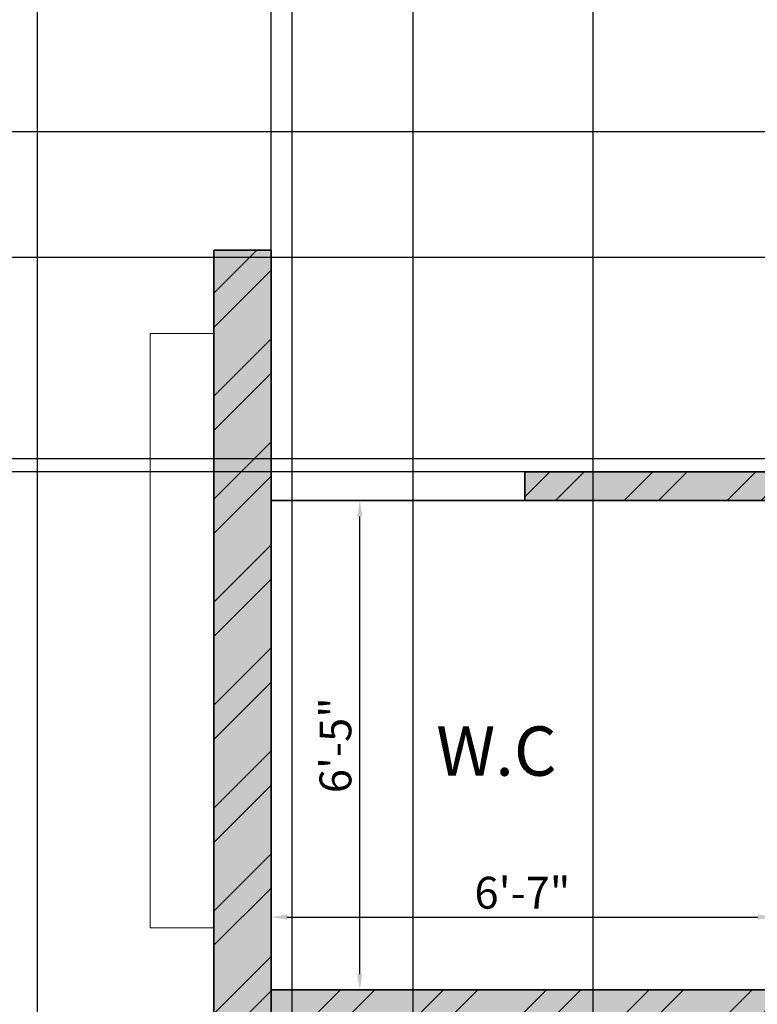
# Model space of a CAD drawing. Units: inches. Extents: x 1804 to 3296, y 909 to 2477.
# Tile 13 of 31: x 2119 to 2235, y 1329 to 1484. Entities that reach past the tile are written whole.
import ezdxf

# ---------------------------------------------------------------- set-up
doc = ezdxf.new("R2010")
doc.units = ezdxf.units.IN
for name, color, linetype, lineweight in [('A-ANNO-DIMS', 2, 'Continuous', 18), ('A-ANNO-TTLB', 156, 'Continuous', 35), ('A-AREA-IDEN', 190, 'Continuous', 18), ('A-WALL-PATT', 10, 'Continuous', 13), ('FUR', 100, 'Continuous', 18), ('WALL', 10, 'Continuous', 35)]:
    doc.layers.add(name, color=color, linetype=linetype, lineweight=lineweight)
doc.styles.get("Standard").update_dxf_attribs({"font": 'arial.ttf'})
doc.dimstyles.new('ISO-25', dxfattribs={"dimtxt": 5, "dimasz": 2.5, "dimexe": 1.25, "dimexo": 0.625, "dimtad": 1, "dimdec": 0, "dimlunit": 4, "dimtxsty": 'Standard', "dimcen": 2.5, "dimadec": 0, "dimazin": 0, "dimtfac": 1, "dimtdec": 0, "dimtmove": 0, "dimatfit": 3, "dimfxl": 1, "dimarcsym": 0})
pattern_1 = [(45, (0, 196.207), (-8.08223, 8.08223), []), (45, (5.388, 196.207), (-8.08223, 8.08223), [])]

# ---------------------------------------------------------------- blocks, each defined once
blk = doc.blocks.new('*D16')
at = {"layer": 'A-ANNO-DIMS', "color": 0, "lineweight": -2, "transparency": 16777216}
for p, q in [((2158.58, 1331.82), (2158.58, 1343.89)), ((2237.56, 1331.82), (2237.56, 1343.89)), ((2161.08, 1342.64), (2235.06, 1342.64))]:
    blk.add_line(p, q, dxfattribs=at)
at = {"layer": 'A-ANNO-DIMS', "color": 0, "lineweight": 100, "transparency": 16777216}
for points in [[(2161.08, 1343.05), (2161.08, 1342.22), (2158.58, 1342.64)], [(2235.06, 1343.05), (2235.06, 1342.22), (2237.56, 1342.64)]]:
    blk.add_solid(points, dxfattribs=at)
at = {"layer": 'Defpoints', "color": 0, "lineweight": 100, "transparency": 16777216}
for p in [(2237.56, 1342.64), (2158.58, 1331.19), (2237.56, 1331.19)]:
    blk.add_point(p, dxfattribs=at)
at = {"layer": 'A-ANNO-DIMS', "color": 0, "transparency": 16777216, "insert": (2198.07, 1345.81), "char_height": 5, "attachment_point": 5}
blk.add_mtext('6\'-7"', dxfattribs=at)
blk = doc.blocks.new('*D17')
at = {"layer": 'A-ANNO-DIMS', "color": 0, "lineweight": -2, "transparency": 16777216}
for p, q in [((2159.2, 1408.06), (2173.77, 1408.06)), ((2172.52, 1333.69), (2172.52, 1405.56)), ((2159.2, 1331.19), (2173.77, 1331.19))]:
    blk.add_line(p, q, dxfattribs=at)
at = {"layer": 'A-ANNO-DIMS', "color": 0, "lineweight": 100, "transparency": 16777216}
for points in [[(2172.1, 1405.56), (2172.93, 1405.56), (2172.52, 1408.06)], [(2172.1, 1333.69), (2172.93, 1333.69), (2172.52, 1331.19)]]:
    blk.add_solid(points, dxfattribs=at)
at = {"layer": 'Defpoints', "color": 0, "lineweight": 100, "transparency": 16777216}
for p in [(2158.58, 1408.06), (2172.52, 1408.06), (2158.58, 1331.19)]:
    blk.add_point(p, dxfattribs=at)
at = {"layer": 'A-ANNO-DIMS', "color": 0, "transparency": 16777216, "insert": (2169.34, 1369.63), "char_height": 5, "attachment_point": 5, "rotation": 90}
blk.add_mtext('6\'-5"', dxfattribs=at)
blk = doc.blocks.new('*D56')
at = {"layer": 'A-ANNO-DIMS', "color": 0, "lineweight": -2, "transparency": 16777216}
for p, q in [((2180.87, 1680.42), (2180.87, 975.89)), ((2268, 1680.42), (2268, 975.89)), ((2183.37, 977.14), (2265.5, 977.14))]:
    blk.add_line(p, q, dxfattribs=at)
at = {"layer": 'A-ANNO-DIMS', "color": 0, "lineweight": 100, "transparency": 16777216}
for points in [[(2183.37, 977.56), (2183.37, 976.72), (2180.87, 977.14)], [(2265.5, 977.56), (2265.5, 976.72), (2268, 977.14)]]:
    blk.add_solid(points, dxfattribs=at)
at = {"layer": 'Defpoints', "color": 0, "lineweight": 100, "transparency": 16777216}
for p in [(2180.87, 1681.04), (2268, 1681.04), (2268, 977.14)]:
    blk.add_point(p, dxfattribs=at)
at = {"layer": 'A-ANNO-DIMS', "color": 0, "transparency": 16777216, "insert": (2224.44, 980.32), "char_height": 5, "attachment_point": 5}
blk.add_mtext('7\'-3"', dxfattribs=at)
blk = doc.blocks.new('*D59')
at = {"layer": 'A-ANNO-DIMS', "color": 0, "lineweight": -2, "transparency": 16777216}
for p, q in [((2121.83, 1590.3), (2121.83, 975.89)), ((2161.83, 1590.3), (2161.83, 975.89)), ((2124.33, 977.14), (2159.33, 977.14))]:
    blk.add_line(p, q, dxfattribs=at)
at = {"layer": 'A-ANNO-DIMS', "color": 0, "lineweight": 100, "transparency": 16777216}
for points in [[(2124.33, 977.56), (2124.33, 976.72), (2121.83, 977.14)], [(2159.33, 977.56), (2159.33, 976.72), (2161.83, 977.14)]]:
    blk.add_solid(points, dxfattribs=at)
at = {"layer": 'Defpoints', "color": 0, "lineweight": 100, "transparency": 16777216}
for p in [(2121.83, 1590.92), (2161.83, 1590.92), (2161.83, 977.14)]:
    blk.add_point(p, dxfattribs=at)
at = {"layer": 'A-ANNO-DIMS', "color": 0, "transparency": 16777216, "insert": (2141.83, 980.32), "char_height": 5, "attachment_point": 5}
blk.add_mtext('3\'-4"', dxfattribs=at)
blk = doc.blocks.new('*D64')
at = {"layer": 'A-ANNO-DIMS', "color": 0, "lineweight": -2, "transparency": 16777216}
for p, q in [((2241.43, 1446.21), (1880.63, 1446.21)), ((1881.88, 1417.08), (1881.88, 1443.71)), ((2241.43, 1414.58), (1880.63, 1414.58))]:
    blk.add_line(p, q, dxfattribs=at)
at = {"layer": 'A-ANNO-DIMS', "color": 0, "lineweight": 100, "transparency": 16777216}
for points in [[(1881.47, 1443.71), (1882.3, 1443.71), (1881.88, 1446.21)], [(1881.47, 1417.08), (1882.3, 1417.08), (1881.88, 1414.58)]]:
    blk.add_solid(points, dxfattribs=at)
at = {"layer": 'Defpoints', "color": 0, "lineweight": 100, "transparency": 16777216}
for p in [(1881.88, 1446.21), (2242.06, 1446.21), (2242.06, 1414.58)]:
    blk.add_point(p, dxfattribs=at)
at = {"layer": 'A-ANNO-DIMS', "color": 0, "transparency": 16777216, "insert": (1878.67, 1430.39), "char_height": 5, "attachment_point": 5, "rotation": 90}
blk.add_mtext('2\'-7 1/2"', dxfattribs=at)
blk = doc.blocks.new('*D66')
at = {"layer": 'A-ANNO-DIMS', "color": 0, "lineweight": -2, "transparency": 16777216}
for p, q in [((2282.03, 1465.94), (1880.63, 1465.94)), ((1881.88, 1415.06), (1881.88, 1463.44)), ((2282.03, 1412.56), (1880.63, 1412.56))]:
    blk.add_line(p, q, dxfattribs=at)
at = {"layer": 'A-ANNO-DIMS', "color": 0, "lineweight": 100, "transparency": 16777216}
for points in [[(1881.47, 1463.44), (1882.3, 1463.44), (1881.88, 1465.94)], [(1881.47, 1415.06), (1882.3, 1415.06), (1881.88, 1412.56)]]:
    blk.add_solid(points, dxfattribs=at)
at = {"layer": 'Defpoints', "color": 0, "lineweight": 100, "transparency": 16777216}
for p in [(1881.88, 1465.94), (2282.65, 1465.94), (2282.65, 1412.56)]:
    blk.add_point(p, dxfattribs=at)
at = {"layer": 'A-ANNO-DIMS', "color": 0, "transparency": 16777216, "insert": (1878.67, 1439.25), "char_height": 5, "attachment_point": 5, "rotation": 90}
blk.add_mtext('4\'-5 1/2"', dxfattribs=at)
blk = doc.blocks.new('*D71')
at = {"layer": 'A-ANNO-DIMS', "color": 0, "lineweight": -2, "transparency": 16777216}
for p, q in [((2158.58, 1272.26), (2158.58, 1874.99)), ((2161.08, 1873.74), (2206.69, 1873.74)), ((2209.19, 1272.26), (2209.19, 1874.99))]:
    blk.add_line(p, q, dxfattribs=at)
at = {"layer": 'A-ANNO-DIMS', "color": 0, "lineweight": 100, "transparency": 16777216}
for points in [[(2161.08, 1874.15), (2161.08, 1873.32), (2158.58, 1873.74)], [(2206.69, 1874.15), (2206.69, 1873.32), (2209.19, 1873.74)]]:
    blk.add_solid(points, dxfattribs=at)
at = {"layer": 'Defpoints', "color": 0, "lineweight": 100, "transparency": 16777216}
for p in [(2209.19, 1873.74), (2158.58, 1271.63), (2209.19, 1271.63)]:
    blk.add_point(p, dxfattribs=at)
at = {"layer": 'A-ANNO-DIMS', "color": 0, "transparency": 16777216, "insert": (2183.88, 1876.95), "char_height": 5, "attachment_point": 5}
blk.add_mtext('4\'-2 1/2"', dxfattribs=at)

msp = doc.modelspace()

# ---------------------------------------------------------------- hatches: boundary and pattern name
at = {"layer": 'A-ANNO-TTLB'}
h = msp.add_hatch(color=256, dxfattribs=at)
h.dxf.hatch_style = 1
h.paths.add_polyline_path([(3294.53, 2476.54), (1803.79, 2476.54), (1805.43, 909.47), (3296.17, 909.47)])
h.paths.add_polyline_path([(1811, 914.33), (1812.79, 2467.54), (3285.53, 2467.54), (3283.74, 914.33)], flags=16)
h.paths.add_polyline_path([(1925.58, 1062.77), (1925.58, 1138.07), (1925.58, 1539.88), (1925.58, 1793.38), (1925.58, 1830.04), (2325.54, 1830.04), (2325.54, 1793.38), (2325.54, 1586.42), (2325.54, 1138.07), (2325.54, 1062.77)], flags=0)
h.paths.add_polyline_path([(1997.22, 1029.4), (2008.85, 1037.96), (2008.85, 1020.84)], flags=0)
h.paths.add_polyline_path([(1934.58, 1138.07), (1934.58, 1147.07), (2078.77, 1147.07), (2078.77, 1138.07), (2060.94, 1138.07)], flags=0)
h.paths.add_polyline_path([(1944.35, 1138.07), (1944.35, 1147.07), (2056.05, 1147.07), (2056.05, 1138.07)], flags=0)
h.paths.add_polyline_path([(2222.24, 1037.96), (2233.87, 1029.4), (2222.24, 1020.84)], flags=0)
h.paths.add_polyline_path([(2061.94, 1139.07), (2061.94, 1146.07), (2077.77, 1146.07), (2077.77, 1139.07)], flags=0)
h.paths.add_polyline_path([(2149.58, 1138.07), (2149.58, 1269.44), (2158.58, 1269.44), (2158.58, 1326.69), (2149.58, 1326.69), (2149.58, 1340.94), (2139.6, 1340.94), (2139.6, 1434.25), (2149.58, 1434.25), (2149.58, 1447.36), (2158.58, 1447.36), (2158.58, 1423.87), (2158.58, 1408.06), (2198.46, 1408.06), (2198.46, 1412.56), (2282.65, 1412.56), (2282.65, 1465.94), (2316.54, 1465.94), (2316.54, 1590.92), (2192.86, 1590.92), (2192.86, 1595.3), (2291.17, 1595.3), (2291.17, 1590.92), (2316.54, 1590.92), (2316.54, 1784.38), (2300.24, 1784.38), (2300.24, 1757.47), (2268, 1757.47), (2268, 1681.04), (2180.87, 1681.04), (2180.87, 1757.47), (2148.63, 1757.47), (2148.63, 1784.38), (2119.08, 1784.38), (2119.08, 1585.58), (2114.58, 1585.58), (2114.58, 1784.38), (2064.11, 1784.38), (2046.28, 1784.38), (2046.28, 1760.38), (1958.58, 1760.38), (1958.58, 1664.38), (1934.58, 1664.38), (1934.58, 1784.38), (1934.58, 1793.38), (2046.28, 1793.38), (2064.11, 1793.38), (2119.08, 1793.38), (2230.78, 1793.38), (2230.78, 1784.38), (2268, 1784.38), (2300.24, 1784.38), (2316.54, 1784.38), (2316.54, 1590.92), (2316.54, 1373.73), (2316.54, 1138.07)], flags=0)
h.paths.add_polyline_path([(2209.19, 1166.63), (2209.19, 1175.63), (2158.58, 1175.63), (2209.19, 1223.63), (2209.19, 1231.63), (2183.88, 1231.63), (2183.88, 1301.66), (2242.59, 1301.66), (2242.59, 1326.69), (2316.54, 1326.69), (2272.59, 1271.63), (2272.59, 1223.63), (2316.54, 1175.63), (2272.59, 1175.63), (2272.59, 1166.63)], flags=0)
h.paths.add_polyline_path([(1947.77, 1345.22), (1947.77, 1457.48), (1991.2, 1457.48), (1991.2, 1451.7), (1991.2, 1352.18), (1991.2, 1345.22)], flags=0)
h.paths.add_polyline_path([(2209.19, 1271.63), (2262.59, 1271.63), (2262.59, 1311.85), (2272.59, 1301.66), (2272.59, 1271.63), (2269.92, 1269.63), (2270.59, 1269.63), (2270.59, 1225.63), (2211.19, 1225.63), (2211.19, 1269.63), (2211.86, 1269.63)], flags=0)
h.paths.add_polyline_path([(2000.34, 1378.21), (2000.34, 1429.71), (2025.22, 1429.71), (2025.22, 1378.21)], flags=0)
h.paths.add_polyline_path([(2001.34, 1379.21), (2001.34, 1428.71), (2024.22, 1428.71), (2024.22, 1379.21)], flags=0)
h.paths.add_polyline_path([(2012.34, 1390.21), (2012.34, 1417.71), (2013.22, 1417.71), (2013.22, 1390.21)], flags=0)
h.paths.add_polyline_path([(2237.56, 1331.19), (2237.56, 1340.18), (2238.62, 1340.18), (2238.62, 1386.84), (2241.04, 1386.84), (2242.06, 1386.84), (2242.06, 1408.06), (2316.54, 1331.19)], flags=0)
h.paths.add_polyline_path([(1953.73, 1464.35), (1953.73, 1498.59), (1981.74, 1498.59), (1981.74, 1464.35)], flags=0)
h.paths.add_polyline_path([(1987.63, 1462.08), (1987.63, 1500.95), (2104.07, 1500.95), (2104.07, 1462.08), (2099.27, 1462.08), (1993.6, 1462.08)], flags=0)
h.paths.add_polyline_path([(1956.06, 1481.47, -1), (1979.41, 1481.47, -1)], flags=0)
edge = h.paths.add_edge_path(flags=0)
edge.add_ellipse((2299.53, 1438.37), major_axis=(0.31, 21.36), ratio=0.670333, start_angle=0, end_angle=360)
h.paths.add_polyline_path([(2297.39, 1438.37, -1), (2301.67, 1438.37, -1)], flags=0)
h.paths.add_polyline_path([(2591.54, 1163.23), (2591.54, 1179.38), (2591.54, 1379.68), (2591.54, 1395.84), (2734.5, 1395.84), (2734.5, 1379.68), (2734.5, 1179.38), (2734.5, 1163.23)], flags=0)
h.paths.add_polyline_path([(2592.54, 1164.23), (2592.54, 1166.23), (2733.5, 1166.23), (2733.5, 1164.23)], flags=0)
h.paths.add_polyline_path([(2592.54, 1180.38), (2592.54, 1378.68), (2733.5, 1378.68), (2733.5, 1180.38)], flags=0)
h.paths.add_polyline_path([(2593.54, 1181.38), (2593.54, 1377.68), (2732.5, 1377.68), (2732.5, 1181.38)], flags=0)
h.paths.add_polyline_path([(2594.54, 1182.38), (2594.54, 1376.68), (2731.5, 1376.68), (2731.5, 1182.38)], flags=0)
h.paths.add_polyline_path([(1936.95, 1697.46), (1936.95, 1736.46), (1955.41, 1736.46), (1955.41, 1697.46)], flags=0)
h.paths.add_polyline_path([(1938.48, 1718.36), (1938.48, 1734.92), (1953.65, 1734.92), (1953.65, 1718.36)], flags=0)
h.paths.add_polyline_path([(1944.75, 1726.64, -1), (1947.37, 1726.64, -1)], flags=0)
h.paths.add_polyline_path([(2592.54, 1394.84), (2733.5, 1394.84), (2733.5, 1392.84), (2592.54, 1392.84)], flags=0)
h.paths.add_polyline_path([(1976.61, 1762.5), (1976.61, 1781.44), (2012.79, 1781.44), (2012.79, 1762.5)], flags=0)
h.paths.add_polyline_path([(1979.57, 1771.97, -1), (1991.39, 1771.97, -1)], flags=0)
h.paths.add_polyline_path([(1995.36, 1771.97, -1), (2007.18, 1771.97, -1)], flags=0)
h.paths.add_polyline_path([(2251.51, 1744.53), (2268, 1730.05), (2251.51, 1730.05)], flags=0)
h.paths.add_polyline_path([(2047.28, 1785.38), (2047.28, 1792.38), (2063.11, 1792.38), (2063.11, 1785.38)], flags=0)
h.paths.add_polyline_path([(2155.08, 1770.92, -1), (2174.42, 1770.92, -1)], flags=0)
h.paths.add_polyline_path([(2188.59, 1758.27), (2188.59, 1772.81), (2222.3, 1772.81), (2222.3, 1758.27)], flags=0)
h.paths.add_polyline_path([(2223.97, 1758.27), (2223.97, 1772.81), (2257.68, 1772.81), (2257.68, 1758.27)], flags=0)
h.paths.add_polyline_path([(2274.45, 1770.92, -1), (2293.8, 1770.92, -1)], flags=0)
h.paths.add_polyline_path([(2591.54, 1582.09), (2591.54, 1782.39), (2734.5, 1782.39), (2734.5, 1582.09)], flags=0)
h.paths.add_polyline_path([(2592.54, 1583.09), (2592.54, 1781.39), (2733.5, 1781.39), (2733.5, 1583.09)], flags=0)
h.paths.add_polyline_path([(2593.54, 1584.09), (2593.54, 1780.39), (2732.5, 1780.39), (2732.5, 1584.09)], flags=0)
h.paths.add_polyline_path([(2594.54, 1585.09), (2594.54, 1779.39), (2731.5, 1779.39), (2731.5, 1585.09)], flags=0)
h.paths.add_polyline_path([(1922.17, 1978.79), (1922.17, 2295.08), (1922.17, 2296.08), (2115.67, 2296.08), (2115.67, 2384.31), (2115.67, 2385.31), (2322.12, 2385.31), (2323.12, 2385.31), (2323.12, 1979.79), (2323.12, 1978.79), (1923.17, 1978.79)], flags=0)
h.paths.add_polyline_path([(1922.17, 1978.79), (1922.17, 2051.31), (1922.17, 2214.86), (1922.17, 2296.08), (2115.67, 2296.08), (2115.67, 2385.31), (2323.12, 2385.31), (2323.12, 2280.42), (2323.12, 1978.79), (2115.67, 1978.79)], flags=0)
h.paths.add_polyline_path([(1923.17, 1979.79), (1923.17, 2050.31), (2115.67, 2050.31), (2115.67, 2051.31), (1923.17, 2051.31), (1923.17, 2213.86), (1923.17, 2214.86), (1923.17, 2295.08), (1990.02, 2295.08), (1990.02, 2214.86), (1991.02, 2214.86), (1991.02, 2295.08), (2115.67, 2295.08), (2115.67, 1979.79), (2116.67, 1979.79), (2116.67, 2304.18), (2116.67, 2384.31), (2322.12, 2384.31), (2322.12, 2280.42), (2322.12, 1979.79), (2115.67, 1979.79)], flags=0)
h.paths.add_polyline_path([(2972.46, 1192.5), (2972.46, 1196.92), (2995.47, 1196.92), (2995.47, 1255.47), (2995.09, 1255.47), (2987.42, 1249.39), (2980.08, 1255.47), (2978.05, 1255.47), (2978.05, 1257.24), (2995.47, 1257.24), (2995.47, 1261.58), (3015.37, 1261.58), (3015.37, 1333.28), (3015.37, 1414.4), (3032.82, 1414.4), (3032.82, 1333.28), (3032.82, 1261.58), (3052.66, 1261.58), (3052.66, 1255.47), (3079.86, 1255.47), (3078.72, 1254.57), (3081.47, 1252.29), (3078.56, 1249.99), (3075.81, 1252.26), (3072.57, 1249.69), (3070.36, 1251.52), (3067.67, 1249.39), (3060.34, 1255.47), (3052.66, 1255.47), (3052.66, 1196.92), (3054.58, 1196.92), (3074, 1196.92), (3074, 1192.5), (3052.66, 1192.5), (2995.47, 1192.5)], flags=0)
h.paths.add_polyline_path([(2490.75, 1979.27), (2490.75, 1980.27), (2596.87, 1980.27), (2596.87, 2051.8), (2596.87, 2052.8), (2596.87, 2216.35), (2596.87, 2297.57), (2717.32, 2297.57), (2710.57, 2305.62), (2724.07, 2305.62), (2717.32, 2297.57), (2782.37, 2297.57), (2782.37, 2395.8), (3006.82, 2395.8), (3006.82, 1981.27), (3093.73, 1981.27), (3093.73, 1980.27), (3047.51, 1980.27), (3046.37, 1979.37), (3049.11, 1977.1), (3046.2, 1974.79), (3043.46, 1977.07), (3040.21, 1974.49), (3038, 1976.32), (3035.32, 1974.2), (3027.98, 1980.27), (2871.83, 1980.27), (2871.83, 1981.27), (2791.37, 1981.27), (2791.37, 2050.8), (2597.87, 2050.8), (2597.87, 1980.27), (2597.87, 1979.27), (2546.27, 1979.27), (2545.12, 1978.37), (2547.87, 1976.1), (2544.96, 1973.79), (2542.22, 1976.07), (2538.97, 1973.49), (2536.76, 1975.32), (2534.07, 1973.2), (2526.74, 1979.27)], flags=0)
h.paths.add_polyline_path([(2597.87, 2051.8), (2606.87, 2051.8), (2606.87, 2258.39), (2597.87, 2258.39), (2597.87, 2296.57), (2606.87, 2296.57), (2606.87, 2262.39), (2782.37, 2262.39), (2782.37, 2296.57), (2790.37, 2296.57), (2790.37, 2262.39), (2791.37, 2262.39), (2791.37, 2305.67), (2791.37, 2385.8), (2996.82, 2385.8), (2996.82, 2339.85), (3006.82, 2339.85), (3006.82, 2250.12), (2997.82, 2250.12), (2997.82, 1981.27), (2996.82, 1981.27), (2872.83, 1981.27), (2872.83, 1991.8), (2871.83, 1991.8), (2871.83, 2050.8), (2790.37, 2050.8), (2597.87, 2050.8)], flags=0)
h.paths.add_polyline_path([(2179.93, 2153.92), (2179.93, 2353.97), (2259.98, 2353.97), (2259.98, 2153.92)], flags=0)
h.paths.add_polyline_path([(2180.93, 2154.92), (2180.93, 2352.97), (2258.98, 2352.97), (2258.98, 2154.92)], flags=0)
h.paths.add_polyline_path([(2960.87, 1608.49), (2960.87, 1753.62), (3070.9, 1753.62), (3070.9, 1608.49)], flags=0)
h.paths.add_polyline_path([(2961.87, 1609.49), (2961.87, 1752.62), (3069.9, 1752.62), (3069.9, 1609.49)], flags=0)
h.paths.add_polyline_path([(2962.87, 1610.49), (2962.87, 1751.62), (3068.9, 1751.62), (3068.9, 1610.49)], flags=0)
h.paths.add_polyline_path([(2963.87, 1611.49), (2963.87, 1750.62), (3067.9, 1750.62), (3067.9, 1611.49)], flags=0)
h.paths.add_polyline_path([(2782.37, 2051.8), (2782.37, 2216.32), (2791.37, 2216.32), (2791.37, 2051.8), (2872.83, 2051.8), (2872.83, 2068.56), (2884.67, 2068.56), (2884.67, 2085.33), (2896.51, 2085.33), (2896.51, 2102.09), (2908.36, 2102.09), (2908.36, 2118.85), (2920.2, 2118.85), (2920.2, 2135.62), (2932.05, 2135.62), (2932.05, 2145.3), (2925.08, 2145.3), (2925.08, 2203.2), (2996.82, 2203.2), (2996.82, 2145.3), (2953.82, 2145.3), (2872.83, 2051.8), (2790.37, 2051.8)], flags=0)
h.paths.add_polyline_path([(2717.32, 2238.65), (2710.57, 2246.7), (2724.07, 2246.7)], flags=0)
h.paths.add_polyline_path([(2003.09, 1122.79), (2017.16, 1122.79), (2017.16, 1138.74), (2003.09, 1138.74)], flags=8)
h.paths.add_polyline_path([(2174.76, 1792.72), (2188.83, 1792.72), (2188.83, 1808.66), (2174.76, 1808.66)], flags=8)
h.paths.add_polyline_path([(1987.95, 1792.51), (2002.02, 1792.51), (2002.02, 1808.45), (1987.95, 1808.45)], flags=8)
h.paths.add_polyline_path([(2148.79, 1289.26), (2160.46, 1289.26), (2160.46, 1305.2), (2148.79, 1305.2)], flags=8)
h.paths.add_polyline_path([(2115.36, 1133.57), (2127.04, 1133.57), (2127.04, 1149.51), (2115.36, 1149.51)], flags=8)
h.paths.add_polyline_path([(2237.58, 1421.48), (2249.25, 1421.48), (2249.25, 1437.43), (2237.58, 1437.43)], flags=8)
h.paths.add_polyline_path([(2134.99, 1584.32), (2146.66, 1584.32), (2146.66, 1600.26), (2134.99, 1600.26)], flags=8)
h.paths.add_polyline_path([(2101.95, 1557.31), (2113.62, 1557.31), (2113.62, 1573.25), (2101.95, 1573.25)], flags=8)
h.paths.add_polyline_path([(2937.85, 1156.77), (3120.41, 1156.77), (3120.41, 1185.72), (2937.85, 1185.72)], flags=8)
h.paths.add_polyline_path([(2980.71, 1786.71), (3050.06, 1786.71), (3050.06, 1802.66), (2980.71, 1802.66)], flags=8)
h.paths.add_polyline_path([(2869.28, 1661.96), (2938.62, 1661.96), (2938.62, 1690.8), (2869.28, 1690.8)], flags=8)
h.paths.add_polyline_path([(3092.27, 1674.86), (3161.62, 1674.86), (3161.62, 1690.8), (3092.27, 1690.8)], flags=8)
h.paths.add_polyline_path([(2980.71, 1674.86), (3050.06, 1674.86), (3050.06, 1690.8), (2980.71, 1690.8)], flags=8)
h.paths.add_polyline_path([(2649.07, 1678.23), (2674.53, 1678.23), (2674.53, 1714.76), (2649.07, 1714.76)], flags=8)
h.paths.add_polyline_path([(2530.84, 1981.63), (2549.13, 1981.63), (2549.13, 1997.57), (2530.84, 1997.57)], flags=8)
h.paths.add_polyline_path([(3031.29, 1981.77), (3049.58, 1981.77), (3049.58, 1997.71), (3031.29, 1997.71)], flags=8)
h.paths.add_polyline_path([(2715.38, 1911.9), (2851.54, 1911.9), (2851.54, 1940.85), (2715.38, 1940.85)], flags=8)
h.paths.add_polyline_path([(2015.23, 1927.36), (2205.42, 1927.36), (2205.42, 1956.3), (2015.23, 1956.3)], flags=8)
h.paths.add_polyline_path([(2671.84, 2057.84), (2702.75, 2057.84), (2702.75, 2073.79), (2671.84, 2073.79)], flags=8)
h.paths.add_polyline_path([(2678.5, 2316.52), (2765.26, 2316.52), (2765.26, 2332.46), (2678.5, 2332.46)], flags=8)
h.paths.add_polyline_path([(2678.48, 2271.96), (2736.41, 2271.96), (2736.41, 2287.9), (2678.48, 2287.9)], flags=8)
h.paths.add_polyline_path([(2019.2, 972.79), (2243.21, 972.79), (2243.21, 1001.74), (2019.2, 1001.74)], flags=8)
h.paths.add_polyline_path([(2097.06, 1021.56), (2132.16, 1021.56), (2132.16, 1037.51), (2097.06, 1037.51)], flags=8)
h.paths.add_polyline_path([(2182.47, 1360.48), (2207.35, 1360.48), (2207.35, 1376.42), (2182.47, 1376.42)], flags=8)
h.paths.add_polyline_path([(2261.12, 1361.77), (2295.01, 1361.77), (2295.01, 1377.71), (2261.12, 1377.71)], flags=8)
h.paths.add_polyline_path([(2245.75, 1511.51), (2278.44, 1511.51), (2278.44, 1527.46), (2245.75, 1527.46)], flags=8)
h.paths.add_polyline_path([(1991.16, 1296.29), (2060.51, 1296.29), (2060.51, 1312.23), (1991.16, 1312.23)], flags=8)
h.paths.add_polyline_path([(2187, 1651.35), (2246.71, 1651.35), (2246.71, 1667.29), (2187, 1667.29)], flags=8)
h.paths.add_polyline_path([(1976.49, 1684.81), (2068.63, 1684.81), (2068.63, 1700.76), (1976.49, 1700.76)], flags=8)
at = {"layer": 'A-WALL-PATT'}
h = msp.add_hatch(color=256, dxfattribs=at)
h.dxf.hatch_style = 1
h.paths.add_polyline_path([(2119.08, 1544.38), (1925.58, 1544.38), (1925.58, 1539.88), (2119.08, 1539.88)])
h.paths.add_polyline_path([(2119.08, 1545.58), (2114.58, 1545.58), (2114.58, 1544.38), (2119.08, 1544.38)])
h.paths.add_polyline_path([(1965.87, 1658.79), (1965.87, 1679.09), (1955.57, 1679.09), (1955.57, 1658.79)], flags=9)
h.paths.add_polyline_path([(2293.18, 1677.29), (2293.18, 1697.58), (2282.88, 1697.58), (2282.88, 1677.29)], flags=9)
h.paths.add_polyline_path([(2271.13, 1545.23), (2287.53, 1545.23), (2287.53, 1555.53), (2271.13, 1555.53)], flags=9)
h.paths.add_polyline_path([(2303.26, 1488.52), (2303.26, 1508.82), (2292.95, 1508.82), (2292.95, 1488.52)], flags=9)
h.paths.add_polyline_path([(2271.13, 1393.15), (2287.53, 1393.15), (2287.53, 1403.45), (2271.13, 1403.45)], flags=9)
h.paths.add_polyline_path([(2306.48, 1361.45), (2306.48, 1377.86), (2296.18, 1377.86), (2296.18, 1361.45)], flags=9)
h.paths.add_polyline_path([(2174.54, 1361.45), (2174.54, 1377.86), (2164.23, 1377.86), (2164.23, 1361.45)], flags=9)
h.paths.add_polyline_path([(1968.21, 1333.34), (1968.21, 1353.64), (1957.91, 1353.64), (1957.91, 1333.34)], flags=9)
h.paths.add_polyline_path([(2003.09, 1122.79), (2017.16, 1122.79), (2017.16, 1138.74), (2003.09, 1138.74)], flags=9)
h.paths.add_polyline_path([(2174.76, 1792.72), (2188.83, 1792.72), (2188.83, 1808.66), (2174.76, 1808.66)], flags=9)
h.paths.add_polyline_path([(1987.95, 1792.51), (2002.02, 1792.51), (2002.02, 1808.45), (1987.95, 1808.45)], flags=9)
h.paths.add_polyline_path([(2148.79, 1289.26), (2160.46, 1289.26), (2160.46, 1305.2), (2148.79, 1305.2)], flags=9)
h.paths.add_polyline_path([(2115.36, 1133.57), (2127.04, 1133.57), (2127.04, 1149.51), (2115.36, 1149.51)], flags=9)
h.paths.add_polyline_path([(2237.58, 1421.48), (2249.25, 1421.48), (2249.25, 1437.43), (2237.58, 1437.43)], flags=9)
h.paths.add_polyline_path([(2134.99, 1584.32), (2146.66, 1584.32), (2146.66, 1600.26), (2134.99, 1600.26)], flags=9)
h.paths.add_polyline_path([(2101.95, 1557.31), (2113.62, 1557.31), (2113.62, 1573.25), (2101.95, 1573.25)], flags=9)
h.paths.add_polyline_path([(2937.85, 1156.77), (3120.41, 1156.77), (3120.41, 1185.72), (2937.85, 1185.72)], flags=9)
h.paths.add_polyline_path([(2980.71, 1786.71), (3050.06, 1786.71), (3050.06, 1802.66), (2980.71, 1802.66)], flags=9)
h.paths.add_polyline_path([(2869.28, 1661.96), (2938.62, 1661.96), (2938.62, 1690.8), (2869.28, 1690.8)], flags=9)
h.paths.add_polyline_path([(3092.27, 1674.86), (3161.62, 1674.86), (3161.62, 1690.8), (3092.27, 1690.8)], flags=9)
h.paths.add_polyline_path([(2980.71, 1674.86), (3050.06, 1674.86), (3050.06, 1690.8), (2980.71, 1690.8)], flags=9)
h.paths.add_polyline_path([(2649.07, 1678.23), (2674.53, 1678.23), (2674.53, 1714.76), (2649.07, 1714.76)], flags=9)
h.paths.add_polyline_path([(2530.84, 1981.63), (2549.13, 1981.63), (2549.13, 1997.57), (2530.84, 1997.57)], flags=9)
h.paths.add_polyline_path([(3031.29, 1981.77), (3049.58, 1981.77), (3049.58, 1997.71), (3031.29, 1997.71)], flags=9)
h.paths.add_polyline_path([(2715.38, 1911.9), (2851.54, 1911.9), (2851.54, 1940.85), (2715.38, 1940.85)], flags=9)
h.paths.add_polyline_path([(2015.23, 1927.36), (2205.42, 1927.36), (2205.42, 1956.3), (2015.23, 1956.3)], flags=9)
h.paths.add_polyline_path([(2671.84, 2057.84), (2702.75, 2057.84), (2702.75, 2073.79), (2671.84, 2073.79)], flags=9)
h.paths.add_polyline_path([(2678.5, 2316.52), (2765.26, 2316.52), (2765.26, 2332.46), (2678.5, 2332.46)], flags=9)
h.paths.add_polyline_path([(2678.48, 2271.96), (2736.41, 2271.96), (2736.41, 2287.9), (2678.48, 2287.9)], flags=9)
h.paths.add_polyline_path([(2019.2, 972.79), (2243.21, 972.79), (2243.21, 1001.74), (2019.2, 1001.74)], flags=9)
h.paths.add_polyline_path([(2097.06, 1021.56), (2132.16, 1021.56), (2132.16, 1037.51), (2097.06, 1037.51)], flags=9)
h.paths.add_polyline_path([(2182.47, 1360.48), (2207.35, 1360.48), (2207.35, 1376.42), (2182.47, 1376.42)], flags=9)
h.paths.add_polyline_path([(2261.12, 1361.77), (2295.01, 1361.77), (2295.01, 1377.71), (2261.12, 1377.71)], flags=9)
h.paths.add_polyline_path([(2245.75, 1511.51), (2278.44, 1511.51), (2278.44, 1527.46), (2245.75, 1527.46)], flags=9)
h.paths.add_polyline_path([(1991.16, 1296.29), (2060.51, 1296.29), (2060.51, 1312.23), (1991.16, 1312.23)], flags=9)
h.paths.add_polyline_path([(2187, 1651.35), (2246.71, 1651.35), (2246.71, 1667.29), (2187, 1667.29)], flags=9)
h.paths.add_polyline_path([(1976.49, 1684.81), (2068.63, 1684.81), (2068.63, 1700.76), (1976.49, 1700.76)], flags=9)
h = msp.add_hatch(color=256, dxfattribs=at)
h.dxf.hatch_style = 1
h.paths.add_polyline_path([(2149.58, 1147.07), (2141.21, 1147.07), (2141.21, 1144.07), (2141.21, 1138.07), (2149.58, 1138.07)])
h.paths.add_polyline_path([(2101.21, 1144.07, -0.01877), (2101.32, 1147.07), (2078.77, 1147.07), (2078.77, 1138.07), (2101.21, 1138.07)])
h.paths.add_polyline_path([(2060.94, 1147.07), (2056.05, 1147.07), (2056.05, 1138.07), (2060.94, 1138.07)])
h.paths.add_polyline_path([(1944.35, 1147.07), (1934.58, 1147.07), (1934.58, 1138.07), (1944.35, 1138.07)])
h.paths.add_polyline_path([(2158.58, 1269.44), (2149.58, 1269.44), (2149.58, 1138.07), (2158.58, 1138.07)])
h.paths.add_polyline_path([(2003.09, 1122.79), (2017.16, 1122.79), (2017.16, 1138.74), (2003.09, 1138.74)], flags=9)
h.paths.add_polyline_path([(2174.76, 1792.72), (2188.83, 1792.72), (2188.83, 1808.66), (2174.76, 1808.66)], flags=9)
h.paths.add_polyline_path([(1987.95, 1792.51), (2002.02, 1792.51), (2002.02, 1808.45), (1987.95, 1808.45)], flags=9)
h.paths.add_polyline_path([(2148.79, 1289.26), (2160.46, 1289.26), (2160.46, 1305.2), (2148.79, 1305.2)], flags=9)
h.paths.add_polyline_path([(2115.36, 1133.57), (2127.04, 1133.57), (2127.04, 1149.51), (2115.36, 1149.51)], flags=9)
h.paths.add_polyline_path([(2237.58, 1421.48), (2249.25, 1421.48), (2249.25, 1437.43), (2237.58, 1437.43)], flags=9)
h.paths.add_polyline_path([(2134.99, 1584.32), (2146.66, 1584.32), (2146.66, 1600.26), (2134.99, 1600.26)], flags=9)
h.paths.add_polyline_path([(2101.95, 1557.31), (2113.62, 1557.31), (2113.62, 1573.25), (2101.95, 1573.25)], flags=9)
h.paths.add_polyline_path([(2937.85, 1156.77), (3120.41, 1156.77), (3120.41, 1185.72), (2937.85, 1185.72)], flags=9)
h.paths.add_polyline_path([(2980.71, 1786.71), (3050.06, 1786.71), (3050.06, 1802.66), (2980.71, 1802.66)], flags=9)
h.paths.add_polyline_path([(2869.28, 1661.96), (2938.62, 1661.96), (2938.62, 1690.8), (2869.28, 1690.8)], flags=9)
h.paths.add_polyline_path([(3092.27, 1674.86), (3161.62, 1674.86), (3161.62, 1690.8), (3092.27, 1690.8)], flags=9)
h.paths.add_polyline_path([(2980.71, 1674.86), (3050.06, 1674.86), (3050.06, 1690.8), (2980.71, 1690.8)], flags=9)
h.paths.add_polyline_path([(2649.07, 1678.23), (2674.53, 1678.23), (2674.53, 1714.76), (2649.07, 1714.76)], flags=9)
h.paths.add_polyline_path([(2530.84, 1981.63), (2549.13, 1981.63), (2549.13, 1997.57), (2530.84, 1997.57)], flags=9)
h.paths.add_polyline_path([(3031.29, 1981.77), (3049.58, 1981.77), (3049.58, 1997.71), (3031.29, 1997.71)], flags=9)
h.paths.add_polyline_path([(2715.38, 1911.9), (2851.54, 1911.9), (2851.54, 1940.85), (2715.38, 1940.85)], flags=9)
h.paths.add_polyline_path([(2015.23, 1927.36), (2205.42, 1927.36), (2205.42, 1956.3), (2015.23, 1956.3)], flags=9)
h.paths.add_polyline_path([(2671.84, 2057.84), (2702.75, 2057.84), (2702.75, 2073.79), (2671.84, 2073.79)], flags=9)
h.paths.add_polyline_path([(2678.5, 2316.52), (2765.26, 2316.52), (2765.26, 2332.46), (2678.5, 2332.46)], flags=9)
h.paths.add_polyline_path([(2678.48, 2271.96), (2736.41, 2271.96), (2736.41, 2287.9), (2678.48, 2287.9)], flags=9)
h.paths.add_polyline_path([(2019.2, 972.79), (2243.21, 972.79), (2243.21, 1001.74), (2019.2, 1001.74)], flags=9)
h.paths.add_polyline_path([(2097.06, 1021.56), (2132.16, 1021.56), (2132.16, 1037.51), (2097.06, 1037.51)], flags=9)
h.paths.add_polyline_path([(2182.47, 1360.48), (2207.35, 1360.48), (2207.35, 1376.42), (2182.47, 1376.42)], flags=9)
h.paths.add_polyline_path([(2261.12, 1361.77), (2295.01, 1361.77), (2295.01, 1377.71), (2261.12, 1377.71)], flags=9)
h.paths.add_polyline_path([(2245.75, 1511.51), (2278.44, 1511.51), (2278.44, 1527.46), (2245.75, 1527.46)], flags=9)
h.paths.add_polyline_path([(1991.16, 1296.29), (2060.51, 1296.29), (2060.51, 1312.23), (1991.16, 1312.23)], flags=9)
h.paths.add_polyline_path([(2187, 1651.35), (2246.71, 1651.35), (2246.71, 1667.29), (2187, 1667.29)], flags=9)
h.paths.add_polyline_path([(1976.49, 1684.81), (2068.63, 1684.81), (2068.63, 1700.76), (1976.49, 1700.76)], flags=9)
h = msp.add_hatch(color=256, dxfattribs=at)
h.dxf.hatch_style = 1
h.paths.add_polyline_path([(2158.58, 1275.49), (2155.29, 1275.49), (2149.58, 1275.49), (2149.58, 1269.44), (2158.58, 1269.44)])
h.paths.add_polyline_path([(2158.58, 1326.69), (2149.58, 1326.69), (2149.58, 1319.33), (2155.29, 1319.33), (2158.58, 1319.33)])
h.paths.add_polyline_path([(2158.58, 1402.2), (2158.58, 1423.87), (2158.58, 1447.36), (2149.58, 1447.36), (2149.58, 1423.87), (2149.58, 1340.94), (2149.58, 1326.69), (2158.58, 1326.69), (2158.58, 1354.23)])
h.paths.add_polyline_path([(1965.87, 1658.79), (1965.87, 1679.09), (1955.57, 1679.09), (1955.57, 1658.79)], flags=9)
h.paths.add_polyline_path([(2293.18, 1677.29), (2293.18, 1697.58), (2282.88, 1697.58), (2282.88, 1677.29)], flags=9)
h.paths.add_polyline_path([(2271.13, 1545.23), (2287.53, 1545.23), (2287.53, 1555.53), (2271.13, 1555.53)], flags=9)
h.paths.add_polyline_path([(2303.26, 1488.52), (2303.26, 1508.82), (2292.95, 1508.82), (2292.95, 1488.52)], flags=9)
h.paths.add_polyline_path([(2271.13, 1393.15), (2287.53, 1393.15), (2287.53, 1403.45), (2271.13, 1403.45)], flags=9)
h.paths.add_polyline_path([(2306.48, 1361.45), (2306.48, 1377.86), (2296.18, 1377.86), (2296.18, 1361.45)], flags=9)
h.paths.add_polyline_path([(2189.9, 1340.62), (2206.31, 1340.62), (2206.31, 1350.92), (2189.9, 1350.92)], flags=9)
h.paths.add_polyline_path([(2174.54, 1361.45), (2174.54, 1377.86), (2164.23, 1377.86), (2164.23, 1361.45)], flags=9)
h.paths.add_polyline_path([(2304.24, 1240.8), (2304.24, 1261.09), (2293.94, 1261.09), (2293.94, 1240.8)], flags=9)
h.paths.add_polyline_path([(2227.19, 1188.73), (2247.49, 1188.73), (2247.49, 1199.03), (2227.19, 1199.03)], flags=9)
h.paths.add_polyline_path([(2181.93, 1144.21), (2181.93, 1160.62), (2171.63, 1160.62), (2171.63, 1144.21)], flags=9)
h.paths.add_polyline_path([(1968.21, 1333.34), (1968.21, 1353.64), (1957.91, 1353.64), (1957.91, 1333.34)], flags=9)
h.paths.add_polyline_path([(2029.78, 1203.53), (2053.95, 1203.53), (2053.95, 1213.83), (2029.78, 1213.83)], flags=9)
h.paths.add_polyline_path([(2576.51, 1671.88), (2576.51, 1692.17), (2566.21, 1692.17), (2566.21, 1671.88)], flags=9)
h.paths.add_polyline_path([(2566.99, 1269.67), (2566.99, 1289.96), (2556.68, 1289.96), (2556.68, 1269.67)], flags=9)
h.paths.add_polyline_path([(2581.85, 1269.17), (2581.85, 1289.46), (2571.54, 1289.46), (2571.54, 1269.17)], flags=9)
h.paths.add_polyline_path([(2650.71, 1409.75), (2674.89, 1409.75), (2674.89, 1420.05), (2650.71, 1420.05)], flags=9)
h.paths.add_polyline_path([(2003.09, 1122.79), (2017.16, 1122.79), (2017.16, 1138.74), (2003.09, 1138.74)], flags=9)
h.paths.add_polyline_path([(2174.76, 1792.72), (2188.83, 1792.72), (2188.83, 1808.66), (2174.76, 1808.66)], flags=9)
h.paths.add_polyline_path([(1987.95, 1792.51), (2002.02, 1792.51), (2002.02, 1808.45), (1987.95, 1808.45)], flags=9)
h.paths.add_polyline_path([(2148.79, 1289.26), (2160.46, 1289.26), (2160.46, 1305.2), (2148.79, 1305.2)], flags=9)
h.paths.add_polyline_path([(2115.36, 1133.57), (2127.04, 1133.57), (2127.04, 1149.51), (2115.36, 1149.51)], flags=9)
h.paths.add_polyline_path([(2237.58, 1421.48), (2249.25, 1421.48), (2249.25, 1437.43), (2237.58, 1437.43)], flags=9)
h.paths.add_polyline_path([(2134.99, 1584.32), (2146.66, 1584.32), (2146.66, 1600.26), (2134.99, 1600.26)], flags=9)
h.paths.add_polyline_path([(2101.95, 1557.31), (2113.62, 1557.31), (2113.62, 1573.25), (2101.95, 1573.25)], flags=9)
h.paths.add_polyline_path([(2937.85, 1156.77), (3120.41, 1156.77), (3120.41, 1185.72), (2937.85, 1185.72)], flags=9)
h.paths.add_polyline_path([(2980.71, 1786.71), (3050.06, 1786.71), (3050.06, 1802.66), (2980.71, 1802.66)], flags=9)
h.paths.add_polyline_path([(2869.28, 1661.96), (2938.62, 1661.96), (2938.62, 1690.8), (2869.28, 1690.8)], flags=9)
h.paths.add_polyline_path([(3092.27, 1674.86), (3161.62, 1674.86), (3161.62, 1690.8), (3092.27, 1690.8)], flags=9)
h.paths.add_polyline_path([(2980.71, 1674.86), (3050.06, 1674.86), (3050.06, 1690.8), (2980.71, 1690.8)], flags=9)
h.paths.add_polyline_path([(2649.07, 1678.23), (2674.53, 1678.23), (2674.53, 1714.76), (2649.07, 1714.76)], flags=9)
h.paths.add_polyline_path([(2530.84, 1981.63), (2549.13, 1981.63), (2549.13, 1997.57), (2530.84, 1997.57)], flags=9)
h.paths.add_polyline_path([(3031.29, 1981.77), (3049.58, 1981.77), (3049.58, 1997.71), (3031.29, 1997.71)], flags=9)
h.paths.add_polyline_path([(2715.38, 1911.9), (2851.54, 1911.9), (2851.54, 1940.85), (2715.38, 1940.85)], flags=9)
h.paths.add_polyline_path([(2015.23, 1927.36), (2205.42, 1927.36), (2205.42, 1956.3), (2015.23, 1956.3)], flags=9)
h.paths.add_polyline_path([(2671.84, 2057.84), (2702.75, 2057.84), (2702.75, 2073.79), (2671.84, 2073.79)], flags=9)
h.paths.add_polyline_path([(2678.5, 2316.52), (2765.26, 2316.52), (2765.26, 2332.46), (2678.5, 2332.46)], flags=9)
h.paths.add_polyline_path([(2678.48, 2271.96), (2736.41, 2271.96), (2736.41, 2287.9), (2678.48, 2287.9)], flags=9)
h.paths.add_polyline_path([(2019.2, 972.79), (2243.21, 972.79), (2243.21, 1001.74), (2019.2, 1001.74)], flags=9)
h.paths.add_polyline_path([(2097.06, 1021.56), (2132.16, 1021.56), (2132.16, 1037.51), (2097.06, 1037.51)], flags=9)
h.paths.add_polyline_path([(2182.47, 1360.48), (2207.35, 1360.48), (2207.35, 1376.42), (2182.47, 1376.42)], flags=9)
h.paths.add_polyline_path([(2261.12, 1361.77), (2295.01, 1361.77), (2295.01, 1377.71), (2261.12, 1377.71)], flags=9)
h.paths.add_polyline_path([(2245.75, 1511.51), (2278.44, 1511.51), (2278.44, 1527.46), (2245.75, 1527.46)], flags=9)
h.paths.add_polyline_path([(1991.16, 1296.29), (2060.51, 1296.29), (2060.51, 1312.23), (1991.16, 1312.23)], flags=9)
h.paths.add_polyline_path([(2187, 1651.35), (2246.71, 1651.35), (2246.71, 1667.29), (2187, 1667.29)], flags=9)
h.paths.add_polyline_path([(1976.49, 1684.81), (2068.63, 1684.81), (2068.63, 1700.76), (1976.49, 1700.76)], flags=9)
h = msp.add_hatch(dxfattribs=at)
h.set_pattern_fill('ANSI32', color=256, scale=1.2)
h.set_pattern_definition(pattern_1)
h.paths.add_polyline_path([(1934.58, 1784.38), (1934.58, 1793.38), (1925.58, 1793.38), (1925.58, 1539.88), (2119.08, 1539.88), (2119.08, 1545.58), (2114.58, 1545.58), (2114.58, 1544.38), (1934.58, 1544.38)])
h.paths.add_polyline_path([(2114.58, 1793.38), (2064.11, 1793.38), (2064.11, 1784.38), (2114.58, 1784.38)], flags=17)
h.paths.add_polyline_path([(2325.54, 1793.38), (2230.78, 1793.38), (2230.78, 1784.38), (2268, 1784.38), (2300.24, 1784.38), (2316.54, 1784.38), (2316.54, 1590.92), (2316.54, 1586.42), (2325.54, 1586.42)])
h.paths.add_polyline_path([(1944.35, 1147.07), (1934.58, 1147.07), (1934.58, 1138.07), (1944.35, 1138.07)])
h.paths.add_polyline_path([(2101.21, 1144.07, -0.01877), (2101.32, 1147.07), (2078.77, 1147.07), (2078.77, 1138.07), (2101.21, 1138.07)])
h.paths.add_polyline_path([(1934.58, 1539.88), (1925.58, 1539.88), (1925.58, 1138.07), (1934.58, 1138.07), (1934.58, 1147.07)])
h.paths.add_polyline_path([(2325.54, 1586.42), (2316.54, 1586.42), (2316.54, 1373.73), (2316.54, 1138.07), (2325.54, 1138.07), (2325.54, 1228.97)])
h.paths.add_polyline_path([(2158.58, 1423.87), (2158.58, 1447.36), (2149.58, 1447.36), (2149.58, 1423.87), (2149.58, 1340.94), (2149.58, 1326.69), (2158.58, 1326.69), (2158.58, 1354.23), (2158.58, 1402.2)])
h.paths.add_polyline_path([(2316.54, 1412.56), (2282.65, 1412.56), (2273.09, 1412.56), (2273.09, 1408.06), (2316.54, 1408.06)])
h.paths.add_polyline_path([(2273.09, 1412.56), (2242.06, 1412.56), (2242.06, 1408.06), (2273.09, 1408.06)])
h.paths.add_polyline_path([(2237.56, 1412.56), (2198.46, 1412.56), (2198.46, 1408.06), (2237.56, 1408.06)])
h.paths.add_polyline_path([(2242.06, 1408.06), (2237.56, 1408.06), (2237.56, 1386.84), (2242.06, 1386.84)])
h.paths.add_polyline_path([(2242.06, 1412.56), (2237.56, 1412.56), (2237.56, 1408.06), (2242.06, 1408.06)])
h.paths.add_polyline_path([(2158.58, 1269.44), (2149.58, 1269.44), (2149.58, 1138.07), (2158.58, 1138.07)])
h.paths.add_polyline_path([(2149.58, 1147.07), (2141.21, 1147.07), (2141.21, 1144.07), (2141.21, 1138.07), (2149.58, 1138.07)])
h.paths.add_polyline_path([(2272.59, 1175.63), (2209.19, 1175.63), (2209.19, 1166.63), (2272.59, 1166.63)])
h.paths.add_polyline_path([(2237.56, 1446.21), (2242.06, 1446.21), (2242.06, 1586.42), (2237.56, 1586.42)])
h.paths.add_polyline_path([(2242.06, 1414.58), (2237.56, 1414.58), (2237.56, 1412.56), (2242.06, 1412.56)])
h = msp.add_hatch(color=256, dxfattribs=at)
h.dxf.hatch_style = 1
h.paths.add_polyline_path([(2114.58, 1793.38), (2064.11, 1793.38), (2064.11, 1784.38), (2114.58, 1784.38)])
h.paths.add_polyline_path([(2119.08, 1793.38), (2114.58, 1793.38), (2114.58, 1585.58), (2119.08, 1585.58)])
h.paths.add_polyline_path([(2325.54, 1793.38), (2230.78, 1793.38), (2230.78, 1784.38), (2268, 1784.38), (2316.54, 1784.38), (2316.54, 1590.92), (2316.54, 1586.42), (2325.54, 1586.42)])
h.paths.add_polyline_path([(2316.54, 1331.19), (2158.58, 1331.19), (2158.58, 1326.69), (2316.54, 1326.69)])
h.paths.add_polyline_path([(2242.06, 1408.06), (2237.56, 1408.06), (2237.56, 1386.84), (2242.06, 1386.84)])
h.paths.add_polyline_path([(2242.06, 1412.56), (2237.56, 1412.56), (2237.56, 1408.06), (2242.06, 1408.06)])
h.paths.add_polyline_path([(2237.56, 1412.56), (2198.46, 1412.56), (2198.46, 1408.06), (2237.56, 1408.06)])
h.paths.add_polyline_path([(2273.09, 1412.56), (2242.06, 1412.56), (2242.06, 1408.06), (2273.09, 1408.06)])
h.paths.add_polyline_path([(2316.54, 1412.56), (2282.65, 1412.56), (2273.09, 1412.56), (2273.09, 1408.06), (2316.54, 1408.06)])
h.paths.add_polyline_path([(2325.54, 1586.42), (2316.54, 1586.42), (2316.54, 1373.73), (2316.54, 1138.07), (2325.54, 1138.07), (2325.54, 1228.97)])
h.paths.add_polyline_path([(2272.59, 1175.63), (2209.19, 1175.63), (2209.19, 1166.63), (2272.59, 1166.63)])
h = msp.add_hatch(dxfattribs=at)
h.set_pattern_fill('ANSI32', color=256, scale=1.2)
h.set_pattern_definition(pattern_1)
h.paths.add_polyline_path([(2316.54, 1331.19), (2158.58, 1331.19), (2158.58, 1326.69), (2316.54, 1326.69)])
h.paths.add_polyline_path([(2242.06, 1340.18), (2237.56, 1340.18), (2237.56, 1331.19), (2242.06, 1331.19)])
h.paths.add_polyline_path([(2242.06, 1408.06), (2237.56, 1408.06), (2237.56, 1386.84), (2242.06, 1386.84)])

# ---------------------------------------------------------------- linework, layer by layer
at = {"layer": 'FUR'}
msp.add_lwpolyline([(2149.58, 1340.94), (2139.6, 1340.94), (2139.6, 1434.25), (2149.58, 1434.25)], close=True, dxfattribs=at)
at = {"layer": 'WALL'}
for p, q in [((2149.58, 1423.87), (2149.58, 1447.36)), ((2149.58, 1447.36), (2158.58, 1447.36)), ((2158.58, 1447.36), (2158.58, 1423.87)), ((2149.58, 1397.11), (2149.58, 1423.87)), ((2158.58, 1398.07), (2158.58, 1423.87)), ((2198.46, 1412.56), (2316.54, 1412.56)), ((2198.46, 1412.56), (2198.46, 1408.06)), ((2158.58, 1408.06), (2316.54, 1408.06)), ((2158.58, 1354.23), (2158.58, 1402.2)), ((2149.58, 1355.19), (2149.58, 1397.11)), ((2149.58, 1326.69), (2149.58, 1355.19)), ((2158.58, 1138.07), (2158.58, 1354.23)), ((2158.58, 1331.19), (2316.54, 1331.19))]:
    msp.add_line(p, q, dxfattribs=at)

# ---------------------------------------------------------------- texts
at = {"layer": 'A-AREA-IDEN', "insert": (2184.53, 1372.57), "char_height": 7.737, "attachment_point": 1}
msp.add_mtext_dynamic_manual_height_columns('W.C', width=163.3261, gutter_width=38.69, heights=[0], dxfattribs=at)

# ---------------------------------------------------------------- dimensions: what is measured, and where the dimension line sits
at = {"layer": 'A-ANNO-DIMS'}
for base, p1, p2, override, picture, middle in [((2209.19, 1873.74), (2158.58, 1271.63), (2209.19, 1271.63), {"dimdec": 1, "dimlfac": 1, "dimrnd": 0, "dimzin": 1, "dimdsep": 46, "dimlunit": 4, "dimfrac": 2}, '*D71', (2183.88, 1876.95)), ((2268, 977.14), (2180.87, 1681.04), (2268, 1681.04), {"dimdec": 1, "dimlfac": 1, "dimrnd": 0, "dimzin": 1, "dimdsep": 46, "dimlunit": 4, "dimfrac": 2}, '*D56', (2224.44, 980.32)), ((2161.83, 977.14), (2121.83, 1590.92), (2161.83, 1590.92), {"dimdec": 1, "dimlfac": 1, "dimrnd": 0, "dimzin": 1, "dimdsep": 46, "dimlunit": 4, "dimfrac": 2}, '*D59', (2141.83, 980.32)), ((2237.56, 1342.64), (2158.58, 1331.19), (2237.56, 1331.19), {"dimclrd": 0, "dimclre": 0, "dimclrt": 0}, '*D16', (2198.07, 1345.81))]:
    dim = msp.add_linear_dim(base=base, p1=p1, p2=p2, dimstyle='ISO-25', override=override, dxfattribs=at)
    dim.commit()
    dim.dimension.update_dxf_attribs({"geometry": picture, "text_midpoint": middle})
for base, p1, p2, override, picture, middle in [((1881.88, 1465.94), (2282.65, 1412.56), (2282.65, 1465.94), {"dimdec": 1, "dimlfac": 1, "dimrnd": 0, "dimzin": 1, "dimdsep": 46, "dimlunit": 4, "dimfrac": 2}, '*D66', (1878.67, 1439.25)), ((1881.88, 1446.21), (2242.06, 1414.58), (2242.06, 1446.21), {"dimdec": 1, "dimlfac": 1, "dimrnd": 0, "dimzin": 1, "dimdsep": 46, "dimlunit": 4, "dimfrac": 2}, '*D64', (1878.67, 1430.39)), ((2172.52, 1408.06), (2158.58, 1331.19), (2158.58, 1408.06), {"dimclrd": 0, "dimclre": 0, "dimclrt": 0}, '*D17', (2169.34, 1369.63))]:
    dim = msp.add_linear_dim(base=base, p1=p1, p2=p2, angle=90, dimstyle='ISO-25', override=override, dxfattribs=at)
    dim.commit()
    dim.dimension.update_dxf_attribs({"geometry": picture, "text_midpoint": middle})

doc.saveas('drawing.dxf')
